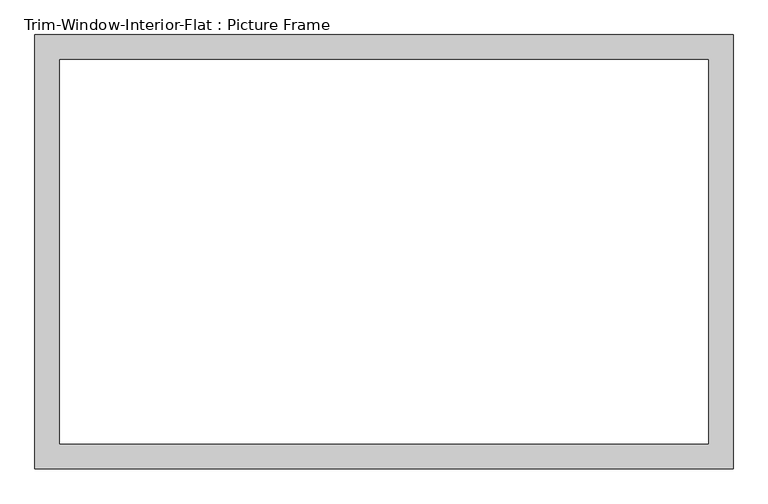
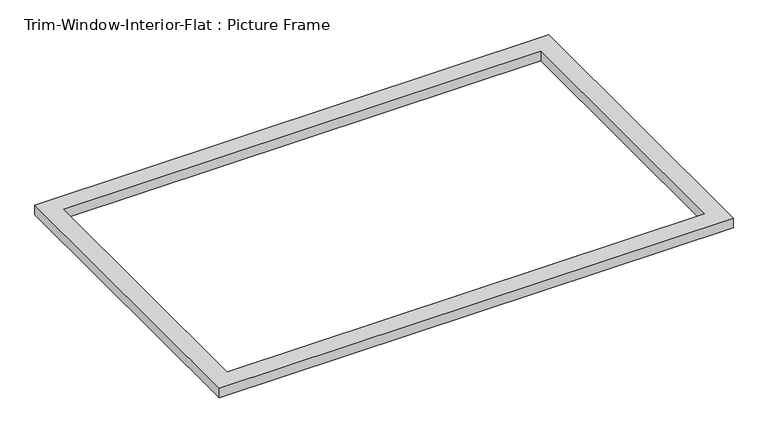
"""IFC4 building model written with IfcOpenShell, lengths in millimetres: proxy geometry, Trim-Window-Interior-Flat : Picture Frame."""

from ifc_helpers import new_model, si_unit, origin, origin_with_axes, place, context, project, spatial, polyline, outline, extrude, source, transform, mapped, element, save


def trim_window_interior_flat_picture_frame_7883d11b(model_context):
    return source(origin(), model_context, "Body", "SweptSolid", [
        extrude(outline(polyline([(806.45, 44.45), (806.45, -958.85), (-806.45, -958.85), (-806.45, 44.45), (806.45, 44.45)]), holes=[polyline([(749.3, -12.7), (-749.3, -12.7), (-749.3, -901.7), (749.3, -901.7), (749.3, -12.7)])]), origin_with_axes(), (0.0, 0.0, 1.0), 31.75),
    ])


if __name__ == "__main__":
    model = new_model("IFC4")
    model_context = context("Model", 3, world=origin())
    ifc_project = project(units=[si_unit("LENGTHUNIT", "METRE", prefix="MILLI")], contexts=[model_context])
    site = spatial("IfcSite", under=ifc_project)
    building = spatial("IfcBuilding", under=site)
    placement = place(None, origin())
    trim_window_interior_flat_picture_frame_shape = trim_window_interior_flat_picture_frame_7883d11b(model_context)
    element("IfcBuildingElementProxy", 1, Name="Trim-Window-Interior-Flat : Picture Frame", ObjectType="Trim-Window-Interior-Flat : Picture Frame", at=placement, inside=building, context=model_context, shape_type="MappedRepresentation", body=[
        mapped(trim_window_interior_flat_picture_frame_shape, transform((0.0, 0.0, 0.0), x_axis=(1.0, 0.0, 0.0), y_axis=(0.0, 1.0, 0.0), z_axis=(0.0, 0.0, 1.0))),
    ])
    save(model, "model.ifc")

# Revit data of these elements
# Type "Trim-Window-Interior-Flat : Picture Frame"
#   Trim Thickness_Picture Frame = 0' - 1 1/4"
#   Trim Width = 0' - 2 1/4"
#   Trim Thickness_with Sill = 0' - 0 3/4"
#   Sill Thickness = 0' - 1 1/4"
#   Opening Width [instance default] = 2' - 0"
#   Opening Height [instance default] = 3' - 0"
#   Default Elevation = 4' - 0"
#   Sill = no
#   Picture Frame = yes
#   Trim Material [instance default] = none
# Element 1 (IfcBuildingElementProxy, "Trim-Window-Interior-Flat : Picture Frame")
#   Opening Width = 5' - 0"
#   Trim Material = Wood - Stained
#   Materials on its faces: "Wood - Stained"
# Materials
#   "Wood - Stained": class "Wood", colour RGB 224 178 126, transparency 0, Cost = 0
